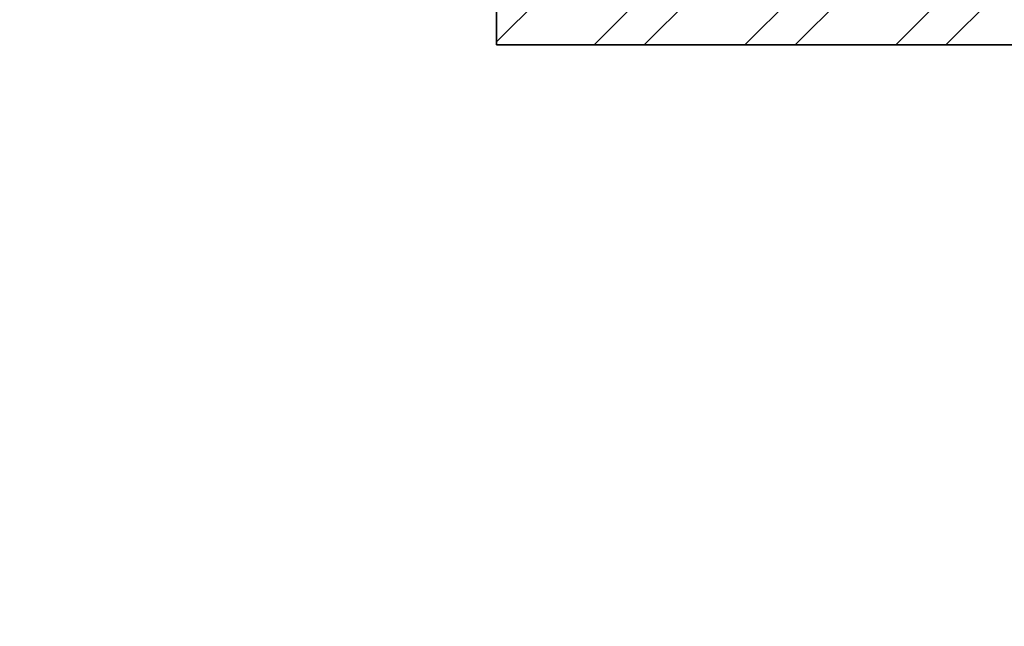
# Model space of a CAD drawing. Units: inches. Extents: x 1885 to 2748, y 783 to 2421.
# Tile 85 of 117: x 2127 to 2215, y 2113 to 2167. Entities that reach past the tile are written whole.
import ezdxf

# ---------------------------------------------------------------- set-up
doc = ezdxf.new("R2010")
doc.units = ezdxf.units.IN
doc.layers.add('A-WALL', color=7, linetype='Continuous', lineweight=35)
doc.layers.add('A-WALL-PATT', color=85, linetype='Continuous', lineweight=13, true_color=0x58ba48)

msp = doc.modelspace()

# ---------------------------------------------------------------- hatches: boundary and pattern name
at = {"layer": 'A-WALL-PATT'}
h = msp.add_hatch(dxfattribs=at)
h.set_pattern_fill('ANSI32', color=256)
h.paths.add_polyline_path([(2007.772, 2318.006), (1980.774, 2318.006), (1980.774, 2281.215), (1985.274, 2281.215), (1985.274, 2313.506), (2007.772, 2313.506), (2007.772, 2315.756)])
h.paths.add_polyline_path([(2094.324, 2318.006), (2067.772, 2318.006), (2067.772, 2313.506), (2094.324, 2313.506), (2094.324, 2315.756)])
h.paths.add_polyline_path([(2131.367, 2315.756), (2131.367, 2318.006), (2131.189, 2318.006), (2112.609, 2318.006), (2112.609, 2313.506), (2117.274, 2313.506), (2117.274, 2255.201), (2121.774, 2255.201), (2121.774, 2313.506), (2131.367, 2313.506)])
h.paths.add_polyline_path([(2190.512, 2318.006), (2155.367, 2318.006), (2155.367, 2313.506), (2169.774, 2313.506), (2169.774, 2229.506), (2121.774, 2229.506), (2121.774, 2233.451), (2119.524, 2233.451), (2117.274, 2233.451), (2117.274, 2201.101), (2121.774, 2201.101), (2121.774, 2225.006), (2169.774, 2225.006), (2169.774, 2165.006), (2306.274, 2165.006), (2306.274, 2066.006), (2310.774, 2066.006), (2344.274, 2066.006), (2486.274, 2066.006), (2486.274, 1886.006), (2483.02, 1886.006), (2483.02, 1881.506), (2486.274, 1881.506), (2486.274, 1880.678), (2490.774, 1880.678), (2490.774, 2070.506), (2344.274, 2070.506), (2310.774, 2070.506), (2310.774, 2165.006), (2310.774, 2173.636), (2308.524, 2173.636), (2306.274, 2173.636), (2306.274, 2169.506), (2174.274, 2169.506), (2174.274, 2313.506), (2190.512, 2313.506), (2190.512, 2315.756)])
h.paths.add_polyline_path([(1985.274, 2221.215), (1980.774, 2221.215), (1980.774, 2165.006), (1992.774, 2165.006), (1992.774, 2141.927), (1997.274, 2141.927), (1997.274, 2165.006), (2117.274, 2165.006), (2117.274, 2163.126), (2121.774, 2163.126), (2121.774, 2172.734), (2119.524, 2172.734), (2117.274, 2172.734), (2117.274, 2169.506), (1985.274, 2169.506)])
h.paths.add_polyline_path([(1997.274, 2105.927), (1992.774, 2105.927), (1992.774, 2070.506), (2016.774, 2070.506), (2016.774, 2059.123), (2019.024, 2059.123), (2021.274, 2059.123), (2021.274, 2070.506), (2117.274, 2070.506), (2117.274, 2022.506), (2114.423, 2022.506), (2114.423, 2018.006), (2123.627, 2018.006), (2123.627, 2020.256), (2123.627, 2022.506), (2121.774, 2022.506), (2121.774, 2142.587), (2119.524, 2142.587), (2117.274, 2142.587), (2117.274, 2075.006), (1997.274, 2075.006)])
h.paths.add_polyline_path([(2092.029, 2020.256), (2092.029, 2022.506), (2021.274, 2022.506), (2021.274, 2035.123), (2016.774, 2035.123), (2016.774, 2018.006), (2016.774, 1978.784), (2021.274, 1978.784), (2021.274, 2018.006), (2092.029, 2018.006)])
h.paths.add_polyline_path([(2260.938, 2022.506), (2153.105, 2022.506), (2153.105, 2020.256), (2153.105, 2018.006), (2155.274, 2018.006), (2155.274, 1886.006), (2107.629, 1886.006), (2107.629, 1881.506), (2182.911, 1881.506), (2182.911, 1883.756), (2182.911, 1886.006), (2159.774, 1886.006), (2159.774, 2018.006), (2260.938, 2018.006), (2260.938, 2020.256)])
h.paths.add_polyline_path([(2047.629, 1883.756), (2047.629, 1886.006), (2021.274, 1886.006), (2021.274, 1918.784), (2019.024, 1918.784), (2016.774, 1918.784), (2016.774, 1881.506), (2047.629, 1881.506)])
h.paths.add_polyline_path([(2306.361, 1883.756), (2306.361, 1886.006), (2296.274, 1886.006), (2296.274, 1982.006), (2316.535, 1982.006), (2316.535, 1984.256), (2316.535, 1986.506), (2296.274, 1986.506), (2296.274, 2022.506), (2289.276, 2022.506), (2289.276, 2018.006), (2291.774, 2018.006), (2291.774, 1886.006), (2242.911, 1886.006), (2242.911, 1881.506), (2306.361, 1881.506)], flags=17)
h.paths.add_polyline_path([(1985.274, 1843.006), (2021.6, 1843.006), (2021.534, 1845.441), (2021.477, 1847.506), (1980.774, 1847.506), (1980.774, 1809.446), (1985.274, 1809.446)])
h.paths.add_polyline_path([(2131.482, 1845.256), (2131.482, 1847.506), (2081.534, 1847.506), (2081.534, 1843.006), (2117.274, 1843.006), (2117.274, 1784.147), (2119.524, 1784.147), (2121.774, 1784.147), (2121.774, 1843.006), (2131.482, 1843.006)])
h.paths.add_polyline_path([(2203.886, 1847.506), (2155.482, 1847.506), (2155.482, 1843.006), (2169.774, 1843.006), (2169.774, 1759.006), (2121.774, 1759.006), (2121.774, 1761.457), (2117.274, 1761.457), (2117.274, 1730.429), (2121.774, 1730.429), (2121.774, 1754.506), (2177.421, 1754.506), (2177.421, 1756.756), (2177.421, 1759.006), (2174.274, 1759.006), (2174.274, 1843.006), (2203.886, 1843.006)])
h.paths.add_polyline_path([(2335.554, 1845.256), (2335.554, 1847.506), (2239.886, 1847.506), (2239.886, 1843.006), (2306.274, 1843.006), (2306.274, 1759.006), (2199.486, 1759.006), (2199.486, 1754.506), (2310.774, 1754.506), (2310.774, 1843.006), (2335.554, 1843.006)])
h.paths.add_polyline_path([(2348.774, 2022.506), (2344.274, 2022.506), (2344.274, 1986.506), (2341.681, 1986.506), (2341.681, 1982.006), (2344.274, 1982.006), (2344.274, 1886.006), (2330.361, 1886.006), (2330.361, 1881.506), (2361.627, 1881.506), (2361.627, 1883.756), (2361.627, 1886.006), (2348.774, 1886.006)], flags=17)
h.paths.add_polyline_path([(2283.251, 2315.756), (2283.251, 2318.006), (2238.512, 2318.006), (2238.512, 2313.506), (2283.251, 2313.506)], flags=17)
h.paths.add_polyline_path([(2363.274, 2348.006), (2388.677, 2348.006), (2388.677, 2350.256), (2388.677, 2352.506), (2358.774, 2352.506), (2358.774, 2348.006), (2358.774, 2318.006), (2344.481, 2318.006), (2344.481, 2313.506), (2358.774, 2313.506), (2358.774, 2229.506), (2310.774, 2229.506), (2310.774, 2231.952), (2306.274, 2231.952), (2306.274, 2205.611), (2310.774, 2205.611), (2310.774, 2225.006), (2358.774, 2225.006), (2358.774, 2211.506), (2452.329, 2211.506), (2452.329, 2213.756), (2452.329, 2216.006), (2363.274, 2216.006), (2363.274, 2318.006)])
h.paths.add_polyline_path([(2310.774, 2313.506), (2320.481, 2313.506), (2320.481, 2315.756), (2320.481, 2318.006), (2302.728, 2318.006), (2302.728, 2313.506), (2306.274, 2313.506), (2306.274, 2251.076), (2310.774, 2251.076)], flags=17)
h.paths.add_polyline_path([(2490.774, 2352.506), (2486.274, 2352.506), (2448.677, 2352.506), (2448.677, 2348.006), (2486.274, 2348.006), (2486.274, 2318.006), (2486.274, 2216.006), (2481.78, 2216.006), (2481.78, 2211.506), (2486.274, 2211.506), (2486.274, 2165.006), (2493.289, 2165.006), (2493.289, 2167.256), (2493.289, 2169.506), (2490.774, 2169.506), (2490.774, 2313.506), (2494.429, 2313.506), (2494.429, 2318.006), (2490.774, 2318.006)])
h.paths.add_polyline_path([(2534.653, 2318.006), (2515.691, 2318.006), (2515.691, 2313.506), (2534.653, 2313.506), (2534.653, 2315.756)])
h.paths.add_polyline_path([(2618.274, 2318.006), (2594.653, 2318.006), (2594.653, 2313.506), (2613.774, 2313.506), (2613.774, 2281.706), (2618.274, 2281.706)])
h.paths.add_polyline_path([(2618.274, 2221.706), (2613.774, 2221.706), (2613.774, 2169.506), (2554.019, 2169.506), (2554.019, 2165.006), (2613.774, 2165.006), (2613.774, 2152.878), (2618.274, 2152.878)])
h.paths.add_polyline_path([(2618.274, 2128.878), (2616.024, 2128.878), (2613.774, 2128.878), (2613.774, 2117.006), (2529.774, 2117.006), (2529.774, 2165.006), (2532.848, 2165.006), (2532.848, 2169.506), (2522.867, 2169.506), (2522.867, 2165.006), (2525.274, 2165.006), (2525.274, 2117.006), (2525.274, 2112.506), (2525.274, 2108.576), (2529.774, 2108.576), (2529.774, 2112.506), (2613.774, 2112.506), (2613.774, 2080.19), (2618.274, 2080.19)])
h.paths.add_polyline_path([(2618.274, 2044.19), (2616.024, 2044.19), (2613.774, 2044.19), (2613.774, 2015.506), (2529.774, 2015.506), (2529.774, 2088.582), (2527.524, 2088.582), (2525.274, 2088.582), (2525.274, 2011.006), (2613.774, 2011.006), (2613.774, 1956.755), (2618.274, 1956.755)])
h.paths.add_polyline_path([(2618.274, 1881.506), (2618.274, 1896.755), (2613.774, 1896.755), (2613.774, 1881.506), (2613.774, 1847.506), (2592.715, 1847.506), (2592.715, 1843.006), (2613.774, 1843.006), (2613.774, 1765.006), (2613.774, 1760.506), (2609.621, 1760.506), (2609.621, 1756.006), (2613.774, 1756.006), (2613.774, 1660.006), (2608.544, 1660.006), (2608.544, 1655.506), (2613.774, 1655.506), (2613.774, 1508.158), (2618.274, 1508.158)])
h.paths.add_polyline_path([(2565.774, 1843.006), (2568.997, 1843.006), (2568.997, 1847.506), (2490.774, 1847.506), (2490.774, 1849.7), (2488.524, 1849.7), (2486.274, 1849.7), (2486.274, 1847.506), (2477.274, 1847.506), (2477.274, 1838.506), (2477.274, 1821.493), (2486.274, 1821.493), (2486.274, 1838.506), (2561.274, 1838.506), (2561.274, 1765.006), (2486.274, 1765.006), (2486.274, 1786.157), (2477.274, 1786.157), (2477.274, 1765.006), (2477.274, 1756.006), (2486.274, 1756.006), (2565.774, 1756.006), (2585.621, 1756.006), (2585.621, 1758.256), (2585.621, 1760.506), (2565.774, 1760.506), (2565.774, 1765.006)])
h.paths.add_polyline_path([(2486.274, 1651.006), (2561.274, 1651.006), (2561.274, 1567.006), (2486.274, 1567.006), (2486.274, 1591.321), (2477.274, 1591.321), (2477.274, 1567.006), (2477.274, 1558.006), (2477.274, 1555.439), (2481.774, 1555.439), (2481.774, 1558.006), (2568.653, 1558.006), (2568.653, 1560.256), (2568.653, 1562.506), (2565.774, 1562.506), (2565.774, 1655.506), (2584.544, 1655.506), (2584.544, 1657.756), (2584.544, 1660.006), (2565.774, 1660.006), (2486.274, 1660.006), (2477.274, 1660.006), (2477.274, 1651.006), (2477.274, 1632.989), (2486.274, 1632.989)])
h.paths.add_polyline_path([(2449.967, 1883.756), (2449.967, 1886.006), (2421.627, 1886.006), (2421.627, 1881.506), (2449.967, 1881.506)], flags=17)
h.paths.add_polyline_path([(2447.274, 1847.506), (2395.554, 1847.506), (2395.554, 1843.006), (2442.774, 1843.006), (2442.774, 1809.27), (2447.274, 1809.27)])
h.paths.add_polyline_path([(1985.274, 1749.446), (1980.774, 1749.446), (1980.774, 1694.504), (1985.274, 1694.504), (1985.274, 1694.506), (1986.897, 1694.506), (1986.897, 1697.78), (1986.897, 1699.006), (1985.274, 1699.006)])
h.paths.add_polyline_path([(2152.774, 1699.006), (2121.774, 1699.006), (2121.774, 1703.668), (2119.524, 1703.668), (2117.274, 1703.668), (2117.274, 1699.006), (2009.219, 1699.006), (2009.219, 1694.506), (2148.274, 1694.506), (2148.274, 1692.631), (2152.774, 1692.631)])
h.paths.add_polyline_path([(2016.274, 1694.506), (2011.774, 1694.506), (2011.774, 1558.006), (2040.806, 1558.006), (2040.806, 1560.256), (2040.806, 1562.506), (2016.274, 1562.506)])
h.paths.add_polyline_path([(2152.774, 1663.017), (2150.524, 1663.017), (2148.274, 1663.017), (2148.274, 1562.506), (2100.806, 1562.506), (2100.806, 1558.006), (2165.119, 1558.006), (2165.119, 1560.256), (2165.119, 1562.506), (2152.774, 1562.506), (2152.774, 1610.506), (2224.774, 1610.506), (2224.774, 1607.99), (2229.274, 1607.99), (2229.274, 1615.006), (2152.774, 1615.006)])
h.paths.add_polyline_path([(2238.613, 1560.256), (2238.613, 1562.506), (2229.274, 1562.506), (2229.274, 1588.756), (2227.024, 1588.763), (2224.774, 1588.771), (2224.774, 1562.506), (2189.119, 1562.506), (2189.119, 1558.006), (2238.613, 1558.006)])
h.paths.add_polyline_path([(2336.024, 1560.256), (2336.024, 1562.506), (2310.774, 1562.506), (2310.774, 1656.347), (2308.524, 1656.347), (2306.274, 1656.347), (2306.274, 1562.506), (2286.613, 1562.506), (2286.613, 1558.006), (2336.024, 1558.006)])
h.paths.add_polyline_path([(2447.274, 1690.968), (2445.024, 1690.968), (2442.774, 1690.968), (2442.774, 1687.006), (2306.274, 1687.006), (2306.274, 1680.75), (2310.774, 1680.75), (2310.774, 1682.506), (2442.774, 1682.506), (2442.774, 1562.506), (2396.024, 1562.506), (2396.024, 1558.006), (2447.274, 1558.006)])
h.paths.add_polyline_path([(2447.274, 1749.27), (2445.024, 1749.27), (2442.774, 1749.27), (2442.774, 1717.232), (2447.274, 1717.232)])
h.paths.add_polyline_path([(2044.674, 1521.756), (2044.674, 1524.006), (2007.274, 1524.006), (2007.274, 1503.49), (2009.524, 1503.49), (2011.774, 1503.49), (2011.774, 1519.506), (2044.674, 1519.506)])
h.paths.add_polyline_path([(2177.969, 1521.756), (2177.969, 1524.006), (2104.674, 1524.006), (2104.674, 1519.506), (2145.774, 1519.506), (2145.774, 1387.506), (2143.37, 1387.506), (2143.37, 1383.006), (2251.585, 1383.006), (2251.585, 1385.256), (2251.585, 1387.506), (2150.274, 1387.506), (2150.274, 1519.506), (2177.969, 1519.506)])
h.paths.add_polyline_path([(2298.704, 1524.006), (2237.969, 1524.006), (2237.969, 1519.506), (2282.274, 1519.506), (2282.274, 1387.506), (2279.683, 1387.506), (2279.683, 1383.006), (2286.774, 1383.006), (2286.774, 1419.006), (2312.451, 1419.006), (2312.451, 1421.256), (2312.451, 1423.506), (2286.774, 1423.506), (2286.774, 1519.506), (2298.704, 1519.506), (2298.704, 1521.722)], flags=17)
h.paths.add_polyline_path([(2361.897, 1521.756), (2361.897, 1524.006), (2322.704, 1524.006), (2322.704, 1519.506), (2334.774, 1519.506), (2334.774, 1423.506), (2331.93, 1423.506), (2331.93, 1419.006), (2334.774, 1419.006), (2334.774, 1387.506), (2334.774, 1383.228), (2339.274, 1383.228), (2339.274, 1387.506), (2339.274, 1519.506), (2361.897, 1519.506)], flags=17)
h.paths.add_polyline_path([(2447.274, 1521.756), (2447.274, 1524.006), (2421.897, 1524.006), (2421.897, 1519.506), (2447.274, 1519.506)], flags=17)
h.paths.add_polyline_path([(2481.774, 1529.6), (2479.524, 1529.6), (2477.274, 1529.6), (2477.274, 1524.006), (2474.489, 1524.006), (2474.489, 1519.506), (2477.274, 1519.506), (2477.274, 1334.506), (2296.774, 1334.506), (2296.774, 1240.506), (2160.274, 1240.506), (2160.274, 1180.506), (2112.274, 1180.506), (2112.274, 1207.692), (2110.024, 1207.692), (2107.774, 1207.692), (2107.774, 1171.609), (2112.274, 1171.609), (2112.274, 1176.006), (2160.274, 1176.006), (2160.274, 1092.006), (2144.221, 1092.006), (2144.221, 1087.506), (2189.497, 1087.506), (2189.497, 1089.756), (2189.497, 1092.006), (2164.774, 1092.006), (2164.774, 1236.006), (2296.774, 1236.006), (2296.774, 1231.912), (2301.274, 1231.912), (2301.274, 1330.006), (2481.774, 1330.006), (2481.774, 1387.506)])
h.paths.add_polyline_path([(2618.274, 1448.158), (2613.774, 1448.158), (2613.774, 1382.506), (2529.774, 1382.506), (2525.274, 1382.506), (2525.274, 1307.062), (2529.774, 1307.062), (2529.774, 1378.006), (2613.774, 1378.006), (2613.774, 1354.988), (2618.274, 1354.988)])
h.paths.add_polyline_path([(2618.274, 1318.988), (2613.774, 1318.988), (2613.774, 1281.006), (2529.774, 1281.006), (2529.774, 1283.786), (2527.524, 1283.786), (2525.274, 1283.786), (2525.274, 1228.506), (2516.794, 1228.506), (2516.794, 1224.006), (2533.484, 1224.006), (2533.484, 1226.256), (2533.484, 1228.506), (2529.774, 1228.506), (2529.774, 1276.506), (2613.774, 1276.506), (2613.774, 1266.02), (2618.274, 1266.02)])
h.paths.add_polyline_path([(2618.274, 1134.964), (2613.774, 1134.964), (2613.774, 1092.006), (2594.545, 1092.006), (2594.545, 1087.506), (2618.274, 1087.506)])
h.paths.add_polyline_path([(2534.545, 1092.006), (2509.765, 1092.006), (2509.765, 1087.506), (2534.545, 1087.506), (2534.545, 1089.756)])
h.paths.add_polyline_path([(2481.274, 1224.006), (2484.117, 1224.006), (2484.117, 1226.256), (2484.117, 1228.506), (2476.774, 1228.506), (2476.774, 1198.506), (2471.61, 1198.506), (2471.61, 1194.006), (2476.774, 1194.006), (2476.774, 1062.006), (2436.894, 1062.006), (2436.894, 1057.506), (2476.774, 1057.506), (2481.274, 1057.506), (2481.274, 1062.006), (2481.274, 1087.506), (2485.354, 1087.506), (2485.354, 1089.756), (2485.354, 1092.006), (2481.274, 1092.006), (2481.274, 1117.506)])
h.paths.add_polyline_path([(2439.898, 1198.506), (2349.274, 1198.506), (2349.274, 1194.006), (2349.274, 1180.506), (2301.274, 1180.506), (2301.274, 1201.896), (2299.024, 1201.896), (2296.774, 1201.896), (2296.774, 1172.335), (2299.024, 1172.335), (2301.274, 1172.335), (2301.274, 1176.006), (2349.274, 1176.006), (2349.274, 1092.006), (2334.452, 1092.006), (2334.452, 1087.506), (2349.274, 1087.506), (2349.274, 1057.506), (2353.774, 1057.506), (2376.894, 1057.506), (2376.894, 1059.756), (2376.894, 1062.006), (2353.774, 1062.006), (2353.774, 1087.506), (2353.774, 1180.506), (2353.774, 1194.006), (2439.898, 1194.006), (2439.898, 1196.256)])
h.paths.add_polyline_path([(2270.596, 1089.756), (2270.596, 1092.006), (2249.497, 1092.006), (2249.497, 1087.506), (2270.596, 1087.506)], flags=17)
h.paths.add_polyline_path([(2310.452, 1092.006), (2301.274, 1092.006), (2301.274, 1153.292), (2296.774, 1153.292), (2296.774, 1092.006), (2293.786, 1092.006), (2293.786, 1087.506), (2310.452, 1087.506), (2310.452, 1089.756)], flags=17)
h.paths.add_polyline_path([(2112.274, 1150.328), (2110.024, 1150.328), (2107.774, 1150.328), (2107.774, 1092.006), (2104.465, 1092.006), (2104.465, 1087.506), (2120.221, 1087.506), (2120.221, 1089.756), (2120.221, 1092.006), (2112.274, 1092.006)])
h.paths.add_polyline_path([(2082.172, 1092.006), (2058.144, 1092.006), (2058.144, 1087.506), (2082.172, 1087.506), (2082.172, 1089.756)])
h.paths.add_polyline_path([(1975.774, 1145.638), (1971.274, 1145.638), (1971.274, 1087.506), (1980.774, 1087.506), (1998.144, 1087.506), (1998.144, 1089.756), (1998.144, 1092.006), (1985.274, 1092.006), (1975.774, 1092.006)])
h.paths.add_polyline_path([(2112.274, 1244.385), (2110.024, 1244.385), (2107.774, 1244.385), (2107.774, 1240.506), (1992.274, 1240.506), (1992.274, 1271.008), (1987.774, 1271.008), (1987.774, 1240.506), (1980.774, 1240.506), (1975.774, 1240.506), (1971.274, 1240.506), (1971.274, 1205.638), (1975.774, 1205.638), (1975.774, 1236.006), (2107.774, 1236.006), (2107.774, 1233.444), (2112.274, 1233.444), (2112.274, 1236.006)])
h.paths.add_polyline_path([(2112.274, 1383.006), (2114.783, 1383.006), (2114.783, 1385.256), (2114.783, 1387.506), (2102.476, 1387.506), (2102.476, 1383.006), (2107.774, 1383.006), (2107.774, 1335.006), (2011.774, 1335.006), (2011.774, 1349.939), (2007.274, 1349.939), (2007.274, 1335.006), (1987.774, 1335.006), (1987.774, 1330.506), (1987.774, 1307.008), (1992.274, 1307.008), (1992.274, 1330.506), (2007.274, 1330.506), (2107.774, 1330.506), (2107.774, 1264.711), (2112.274, 1264.711)])
h.paths.add_polyline_path([(2077.857, 1387.506), (2011.774, 1387.506), (2011.774, 1390.036), (2009.524, 1390.036), (2007.274, 1390.036), (2007.274, 1373.939), (2011.774, 1373.939), (2011.774, 1383.006), (2077.857, 1383.006)])
h.paths.add_polyline_path([(2011.774, 1443.49), (2007.274, 1443.49), (2007.274, 1410.248), (2011.774, 1410.248)])

# ---------------------------------------------------------------- linework, layer by layer
at = {"layer": 'A-WALL'}
for p, q in [((2169.774, 2225.006), (2169.774, 2165.006)), ((2169.774, 2165.006), (2306.274, 2165.006))]:
    msp.add_line(p, q, dxfattribs=at)

doc.saveas('drawing.dxf')
